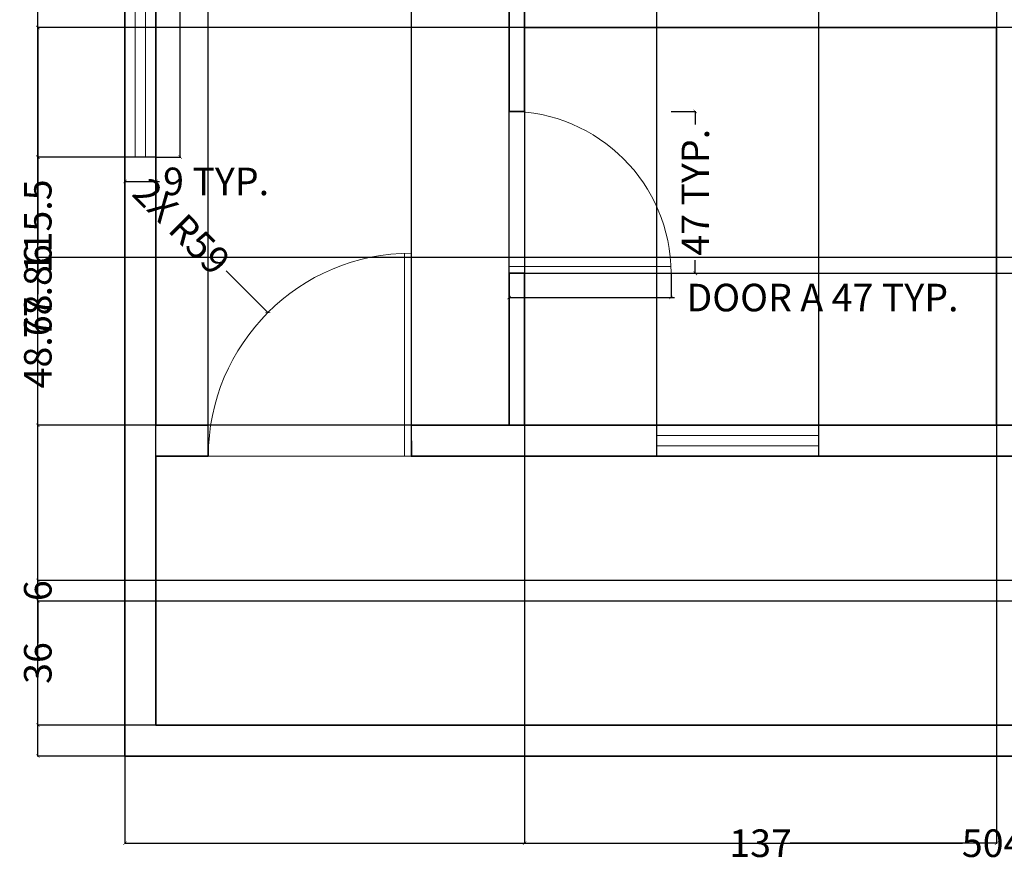
# Model space of a CAD drawing. Units: inches. Extents: x 878 to 1443, y 634 to 1188.
# Tile 1 of 5: x 878 to 1164, y 634 to 878. Entities that reach past the tile are written whole.
import ezdxf

# ---------------------------------------------------------------- set-up
doc = ezdxf.new("R2010")
doc.units = ezdxf.units.IN
doc.header["$MEASUREMENT"] = 0
doc.layers.add('A-ANNO-DIMS', color=2, linetype='Continuous', lineweight=18)
doc.layers.add('A-WALL', color=7, linetype='Continuous', lineweight=35)
doc.layers.add('A-DOOR', color=41, linetype='Continuous', lineweight=18, true_color=0xf4ee51)
doc.layers.add('A-GLAZ', color=152, linetype='Continuous', lineweight=18, true_color=0x2776bb)
doc.styles.get("Standard").update_dxf_attribs({"font": 'arial.ttf'})
doc.dimstyles.get("Standard").update_dxf_attribs({"dimtxt": 8, "dimasz": 1, "dimexe": 0.18, "dimexo": 0.0625, "dimgap": 0.09, "dimtad": 0, "dimdec": 4, "dimzin": 0, "dimdsep": 46, "dimlunit": 3, "dimtxsty": 'Standard', "dimblk": 'ARCHTICK', "dimcen": 0.09, "dimclrd": 6, "dimclre": 5, "dimclrt": 140, "dimadec": 0, "dimazin": 0, "dimtfac": 1, "dimtdec": 4, "dimtofl": 0, "dimtmove": 0, "dimatfit": 3, "dimfxl": 1, "dimtolj": 1, "dimtzin": 0, "dimarcsym": 0})

# ---------------------------------------------------------------- blocks, each defined once
blk = doc.blocks.new('WIN-47IN')
for p, q in [((9, 47), (0, 47)), ((0, 47), (0, 0)), ((3, 0), (3, 47)), ((6, 0), (6, 47)), ((9, 0), (9, 47)), ((0, 0), (9, 0))]:
    blk.add_line(p, q)
blk = doc.blocks.new('DOOR-47IN')
for p, q in [((0, 47), (0, 0)), ((0, 2), (46.96, 2)), ((0, 0), (47, 0))]:
    blk.add_line(p, q)
blk.add_arc((0, 0), 47, 0, 90)
blk = doc.blocks.new('DOOR-59IN')
for p, q in [((57, 0), (57, 58.97)), ((59, 0), (59, 59)), ((0, 0), (59, 0))]:
    blk.add_line(p, q)
blk.add_arc((59, 0), 59, 90, 180)
blk = doc.blocks.new('_ArchTick')
at = {"color": 0, "linetype": 'ByBlock', "const_width": 0.15}
blk.add_lwpolyline([(-0.5, -0.5), (0.5, 0.5)], dxfattribs=at)
blk = doc.blocks.new('*D9')
at = {"layer": 'A-ANNO-DIMS', "color": 6, "lineweight": -2, "transparency": 16777216}
for p, q in [((924.95, 885.33), (924.95, 886.33)), ((924.95, 838.33), (924.95, 885.33))]:
    blk.add_line(p, q, dxfattribs=at)
at = {"layer": 'A-ANNO-DIMS', "color": 5, "lineweight": -2, "transparency": 16777216}
for p, q in [((917.96, 885.33), (925.13, 885.33)), ((917.96, 838.33), (925.13, 838.33))]:
    blk.add_line(p, q, dxfattribs=at)
at = {"layer": 'Defpoints', "color": 0, "lineweight": -2, "transparency": 16777216}
for p in [(917.9, 885.33), (924.95, 885.33), (917.9, 838.33)]:
    blk.add_point(p, dxfattribs=at)
at = {"layer": 'A-ANNO-DIMS', "color": 6, "lineweight": -2, "transparency": 16777216}
for p, rotation in [((924.95, 885.33), 90), ((924.95, 838.33), 270)]:
    blk.add_blockref('_ArchTick', p, dxfattribs=dict(at, rotation=rotation))
at = {"layer": 'A-ANNO-DIMS', "color": 140, "transparency": 16777216, "insert": (924.95, 937.4), "char_height": 8, "attachment_point": 5, "rotation": 90}
blk.add_mtext('\\A1;WINDOW A 47 TYP.', dxfattribs=at)
blk = doc.blocks.new('*D10')
at = {"layer": 'A-ANNO-DIMS', "color": 5, "lineweight": -2, "transparency": 16777216}
for p, q in [((908.9, 838.26), (908.9, 831.1)), ((917.9, 838.26), (917.9, 831.1))]:
    blk.add_line(p, q, dxfattribs=at)
at = {"layer": 'A-ANNO-DIMS', "color": 6, "lineweight": -2, "transparency": 16777216}
for p, q in [((908.9, 831.28), (917.9, 831.28)), ((917.9, 831.28), (918.9, 831.28))]:
    blk.add_line(p, q, dxfattribs=at)
at = {"layer": 'Defpoints', "color": 0, "lineweight": -2, "transparency": 16777216}
for p in [(908.9, 838.33), (917.9, 838.33), (917.9, 831.28)]:
    blk.add_point(p, dxfattribs=at)
at = {"layer": 'A-ANNO-DIMS', "color": 6, "lineweight": -2, "transparency": 16777216, "rotation": 180}
blk.add_blockref('_ArchTick', (908.9, 831.28), dxfattribs=at)
at = {"layer": 'A-ANNO-DIMS', "color": 6, "lineweight": -2, "transparency": 16777216}
blk.add_blockref('_ArchTick', (917.9, 831.28), dxfattribs=at)
at = {"layer": 'A-ANNO-DIMS', "color": 140, "transparency": 16777216, "insert": (935.35, 831.28), "char_height": 8, "attachment_point": 5}
blk.add_mtext('\\A1;9 TYP.', dxfattribs=at)
blk = doc.blocks.new('*D15')
at = {"layer": 'A-ANNO-DIMS', "color": 5, "lineweight": -2, "transparency": 16777216}
for p, q in [((1020.4, 804.54), (1020.4, 797.38)), ((1067.4, 804.54), (1067.4, 797.38))]:
    blk.add_line(p, q, dxfattribs=at)
at = {"layer": 'A-ANNO-DIMS', "color": 6, "lineweight": -2, "transparency": 16777216}
for p, q in [((1020.4, 797.56), (1067.4, 797.56)), ((1067.4, 797.56), (1068.4, 797.56))]:
    blk.add_line(p, q, dxfattribs=at)
at = {"layer": 'Defpoints', "color": 0, "lineweight": -2, "transparency": 16777216}
for p in [(1020.4, 804.61), (1067.4, 804.61), (1067.4, 797.56)]:
    blk.add_point(p, dxfattribs=at)
at = {"layer": 'A-ANNO-DIMS', "color": 6, "lineweight": -2, "transparency": 16777216, "rotation": 180}
blk.add_blockref('_ArchTick', (1020.4, 797.56), dxfattribs=at)
at = {"layer": 'A-ANNO-DIMS', "color": 6, "lineweight": -2, "transparency": 16777216}
blk.add_blockref('_ArchTick', (1067.4, 797.56), dxfattribs=at)
at = {"layer": 'A-ANNO-DIMS', "color": 140, "transparency": 16777216, "insert": (1111.36, 797.56), "char_height": 8, "attachment_point": 5}
blk.add_mtext('\\A1;DOOR A 47 TYP.', dxfattribs=at)
blk = doc.blocks.new('*D16')
at = {"layer": 'A-ANNO-DIMS', "color": 5, "lineweight": -2, "transparency": 16777216}
for p, q in [((1067.46, 851.61), (1074.63, 851.61)), ((1067.46, 804.61), (1074.63, 804.61))]:
    blk.add_line(p, q, dxfattribs=at)
at = {"layer": 'A-ANNO-DIMS', "color": 6, "lineweight": -2, "transparency": 16777216}
for p, q in [((1074.45, 851.61), (1074.45, 847.83)), ((1074.45, 804.61), (1074.45, 808.39))]:
    blk.add_line(p, q, dxfattribs=at)
at = {"layer": 'Defpoints', "color": 0, "lineweight": -2, "transparency": 16777216}
for p in [(1067.4, 851.61), (1074.45, 851.61), (1067.4, 804.61)]:
    blk.add_point(p, dxfattribs=at)
at = {"layer": 'A-ANNO-DIMS', "color": 6, "lineweight": -2, "transparency": 16777216}
for p, rotation in [((1074.45, 851.61), 90), ((1074.45, 804.61), 270)]:
    blk.add_blockref('_ArchTick', p, dxfattribs=dict(at, rotation=rotation))
at = {"layer": 'A-ANNO-DIMS', "color": 140, "transparency": 16777216, "insert": (1074.45, 828.11), "char_height": 8, "attachment_point": 5, "rotation": 90}
blk.add_mtext('\\A1;47 TYP.', dxfattribs=at)
blk = doc.blocks.new('*D21')
at = {"layer": 'A-ANNO-DIMS', "color": 5, "lineweight": -2, "transparency": 16777216}
for p, q in [((908.9, 664.41), (908.9, 638.98)), ((1412.9, 664.41), (1412.9, 638.98))]:
    blk.add_line(p, q, dxfattribs=at)
at = {"layer": 'A-ANNO-DIMS', "color": 6, "lineweight": -2, "transparency": 16777216}
for p, q in [((908.9, 639.16), (1151.99, 639.16)), ((1412.9, 639.16), (1169.81, 639.16))]:
    blk.add_line(p, q, dxfattribs=at)
at = {"layer": 'Defpoints', "color": 0, "lineweight": -2, "transparency": 16777216}
for p in [(908.9, 664.47), (1412.9, 664.47), (1412.9, 639.16)]:
    blk.add_point(p, dxfattribs=at)
at = {"layer": 'A-ANNO-DIMS', "color": 6, "lineweight": -2, "transparency": 16777216, "rotation": 180}
blk.add_blockref('_ArchTick', (908.9, 639.16), dxfattribs=at)
at = {"layer": 'A-ANNO-DIMS', "color": 6, "lineweight": -2, "transparency": 16777216}
blk.add_blockref('_ArchTick', (1412.9, 639.16), dxfattribs=at)
at = {"layer": 'A-ANNO-DIMS', "color": 140, "transparency": 16777216, "insert": (1160.9, 639.16), "char_height": 8, "attachment_point": 5}
blk.add_mtext('\\A1;504', dxfattribs=at)
blk = doc.blocks.new('*D22')
at = {"layer": 'A-ANNO-DIMS', "color": 5, "lineweight": -2, "transparency": 16777216}
for p, q in [((908.84, 1120.47), (883.41, 1120.47)), ((908.84, 664.47), (883.41, 664.47))]:
    blk.add_line(p, q, dxfattribs=at)
at = {"layer": 'A-ANNO-DIMS', "color": 6, "lineweight": -2, "transparency": 16777216}
for p, q in [((883.59, 1120.47), (883.59, 901.56)), ((883.59, 664.47), (883.59, 883.38))]:
    blk.add_line(p, q, dxfattribs=at)
at = {"layer": 'Defpoints', "color": 0, "lineweight": -2, "transparency": 16777216}
for p in [(883.59, 1120.47), (908.9, 1120.47), (908.9, 664.47)]:
    blk.add_point(p, dxfattribs=at)
at = {"layer": 'A-ANNO-DIMS', "color": 6, "lineweight": -2, "transparency": 16777216}
for p, rotation in [((883.59, 1120.47), 90), ((883.59, 664.47), 270)]:
    blk.add_blockref('_ArchTick', p, dxfattribs=dict(at, rotation=rotation))
at = {"layer": 'A-ANNO-DIMS', "color": 140, "transparency": 16777216, "insert": (883.59, 892.47), "char_height": 8, "attachment_point": 5, "rotation": 90}
blk.add_mtext('\\A1;456', dxfattribs=at)
blk = doc.blocks.new('*D28')
at = {"layer": 'A-ANNO-DIMS', "color": 5, "lineweight": -2, "transparency": 16777216}
for p, q in [((917.84, 838.33), (883.41, 838.33)), ((917.84, 760.47), (883.41, 760.47))]:
    blk.add_line(p, q, dxfattribs=at)
at = {"layer": 'A-ANNO-DIMS', "color": 6, "lineweight": -2, "transparency": 16777216}
for p, q in [((883.59, 838.33), (883.59, 812.95)), ((883.59, 760.47), (883.59, 785.85))]:
    blk.add_line(p, q, dxfattribs=at)
at = {"layer": 'Defpoints', "color": 0, "lineweight": -2, "transparency": 16777216}
for p in [(883.59, 838.33), (917.9, 838.33), (917.9, 760.47)]:
    blk.add_point(p, dxfattribs=at)
at = {"layer": 'A-ANNO-DIMS', "color": 6, "lineweight": -2, "transparency": 16777216}
for p, rotation in [((883.59, 838.33), 90), ((883.59, 760.47), 270)]:
    blk.add_blockref('_ArchTick', p, dxfattribs=dict(at, rotation=rotation))
at = {"layer": 'A-ANNO-DIMS', "color": 140, "transparency": 16777216, "insert": (883.59, 799.4), "char_height": 8, "attachment_point": 5, "rotation": 90}
blk.add_mtext('\\A1;77.86', dxfattribs=at)
blk = doc.blocks.new('*D33')
at = {"layer": 'A-ANNO-DIMS', "color": 5, "lineweight": -2, "transparency": 16777216}
for p, q in [((917.9, 760.53), (917.9, 1145.96)), ((1020.4, 760.53), (1020.4, 1145.96))]:
    blk.add_line(p, q, dxfattribs=at)
at = {"layer": 'A-ANNO-DIMS', "color": 6, "lineweight": -2, "transparency": 16777216}
for p, q in [((917.9, 1145.78), (955.91, 1145.78)), ((1020.4, 1145.78), (982.39, 1145.78))]:
    blk.add_line(p, q, dxfattribs=at)
at = {"layer": 'Defpoints', "color": 0, "lineweight": -2, "transparency": 16777216}
for p in [(1020.4, 1145.78), (917.9, 760.47), (1020.4, 760.47)]:
    blk.add_point(p, dxfattribs=at)
at = {"layer": 'A-ANNO-DIMS', "color": 6, "lineweight": -2, "transparency": 16777216, "rotation": 180}
blk.add_blockref('_ArchTick', (917.9, 1145.78), dxfattribs=at)
at = {"layer": 'A-ANNO-DIMS', "color": 6, "lineweight": -2, "transparency": 16777216}
blk.add_blockref('_ArchTick', (1020.4, 1145.78), dxfattribs=at)
at = {"layer": 'A-ANNO-DIMS', "color": 140, "transparency": 16777216, "insert": (969.15, 1145.78), "char_height": 8, "attachment_point": 5}
blk.add_mtext('\\A1;102.5', dxfattribs=at)
blk = doc.blocks.new('*D34')
at = {"layer": 'A-ANNO-DIMS', "color": 5, "lineweight": -2, "transparency": 16777216}
for p, q in [((1024.9, 1111.41), (1024.9, 638.98)), ((1161.9, 1111.41), (1161.9, 638.98))]:
    blk.add_line(p, q, dxfattribs=at)
at = {"layer": 'A-ANNO-DIMS', "color": 6, "lineweight": -2, "transparency": 16777216}
for p, q in [((1024.9, 639.16), (1084.85, 639.16)), ((1161.9, 639.16), (1101.95, 639.16))]:
    blk.add_line(p, q, dxfattribs=at)
at = {"layer": 'Defpoints', "color": 0, "lineweight": -2, "transparency": 16777216}
for p in [(1024.9, 1111.47), (1161.9, 1111.47), (1161.9, 639.16)]:
    blk.add_point(p, dxfattribs=at)
at = {"layer": 'A-ANNO-DIMS', "color": 6, "lineweight": -2, "transparency": 16777216, "rotation": 180}
blk.add_blockref('_ArchTick', (1024.9, 639.16), dxfattribs=at)
at = {"layer": 'A-ANNO-DIMS', "color": 6, "lineweight": -2, "transparency": 16777216}
blk.add_blockref('_ArchTick', (1161.9, 639.16), dxfattribs=at)
at = {"layer": 'A-ANNO-DIMS', "color": 140, "transparency": 16777216, "insert": (1093.4, 639.16), "char_height": 8, "attachment_point": 5}
blk.add_mtext('\\A1;137', dxfattribs=at)
blk = doc.blocks.new('*D38')
at = {"layer": 'A-ANNO-DIMS', "color": 5, "lineweight": -2, "transparency": 16777216}
for p, q in [((1403.84, 875.97), (883.41, 875.97)), ((1403.84, 760.47), (883.41, 760.47))]:
    blk.add_line(p, q, dxfattribs=at)
at = {"layer": 'A-ANNO-DIMS', "color": 6, "lineweight": -2, "transparency": 16777216}
for p, q in [((883.59, 875.97), (883.59, 831.46)), ((883.59, 760.47), (883.59, 804.98))]:
    blk.add_line(p, q, dxfattribs=at)
at = {"layer": 'Defpoints', "color": 0, "lineweight": -2, "transparency": 16777216}
for p in [(1403.9, 875.97), (883.59, 760.47), (1403.9, 760.47)]:
    blk.add_point(p, dxfattribs=at)
at = {"layer": 'A-ANNO-DIMS', "color": 6, "lineweight": -2, "transparency": 16777216}
for p, rotation in [((883.59, 875.97), 90), ((883.59, 760.47), 270)]:
    blk.add_blockref('_ArchTick', p, dxfattribs=dict(at, rotation=rotation))
at = {"layer": 'A-ANNO-DIMS', "color": 140, "transparency": 16777216, "insert": (883.59, 818.22), "char_height": 8, "attachment_point": 5, "rotation": 90}
blk.add_mtext('\\A1;115.5', dxfattribs=at)
blk = doc.blocks.new('*D44')
at = {"layer": 'A-ANNO-DIMS', "color": 5, "lineweight": -2, "transparency": 16777216}
for p, q in [((917.9, 751.53), (917.9, 1145.96)), ((933.09, 751.53), (933.09, 1145.96))]:
    blk.add_line(p, q, dxfattribs=at)
at = {"layer": 'A-ANNO-DIMS', "color": 6, "lineweight": -2, "transparency": 16777216}
for p, q in [((917.9, 1145.78), (933.09, 1145.78)), ((933.09, 1145.78), (934.09, 1145.78))]:
    blk.add_line(p, q, dxfattribs=at)
at = {"layer": 'Defpoints', "color": 0, "lineweight": -2, "transparency": 16777216}
for p in [(933.09, 1145.78), (917.9, 751.47), (933.09, 751.47)]:
    blk.add_point(p, dxfattribs=at)
at = {"layer": 'A-ANNO-DIMS', "color": 6, "lineweight": -2, "transparency": 16777216, "rotation": 180}
blk.add_blockref('_ArchTick', (917.9, 1145.78), dxfattribs=at)
at = {"layer": 'A-ANNO-DIMS', "color": 6, "lineweight": -2, "transparency": 16777216}
blk.add_blockref('_ArchTick', (933.09, 1145.78), dxfattribs=at)
at = {"layer": 'A-ANNO-DIMS', "color": 140, "transparency": 16777216, "insert": (950.4, 1145.78), "char_height": 8, "attachment_point": 5}
blk.add_mtext('\\A1;15.187', dxfattribs=at)
blk = doc.blocks.new('*D45')
at = {"layer": 'A-ANNO-DIMS', "color": 5, "lineweight": -2, "transparency": 16777216}
for p, q in [((992.09, 751.53), (992.09, 1145.96)), ((1063.3, 751.53), (1063.3, 1145.96))]:
    blk.add_line(p, q, dxfattribs=at)
at = {"layer": 'A-ANNO-DIMS', "color": 6, "lineweight": -2, "transparency": 16777216}
for p, q in [((992.09, 1145.78), (1014.18, 1145.78)), ((1063.3, 1145.78), (1041.21, 1145.78))]:
    blk.add_line(p, q, dxfattribs=at)
at = {"layer": 'Defpoints', "color": 0, "lineweight": -2, "transparency": 16777216}
for p in [(1063.3, 1145.78), (992.09, 751.47), (1063.3, 751.47)]:
    blk.add_point(p, dxfattribs=at)
at = {"layer": 'A-ANNO-DIMS', "color": 6, "lineweight": -2, "transparency": 16777216, "rotation": 180}
blk.add_blockref('_ArchTick', (992.09, 1145.78), dxfattribs=at)
at = {"layer": 'A-ANNO-DIMS', "color": 6, "lineweight": -2, "transparency": 16777216}
blk.add_blockref('_ArchTick', (1063.3, 1145.78), dxfattribs=at)
at = {"layer": 'A-ANNO-DIMS', "color": 140, "transparency": 16777216, "insert": (1027.69, 1145.78), "char_height": 8, "attachment_point": 5}
blk.add_mtext('\\A1;71.22', dxfattribs=at)
blk = doc.blocks.new('*D46')
at = {"layer": 'A-ANNO-DIMS', "color": 5, "lineweight": -2, "transparency": 16777216}
for p, q in [((1110.3, 751.53), (1110.3, 1145.96)), ((1172.39, 751.53), (1172.39, 1145.96))]:
    blk.add_line(p, q, dxfattribs=at)
at = {"layer": 'A-ANNO-DIMS', "color": 6, "lineweight": -2, "transparency": 16777216}
for p, q in [((1110.3, 1145.78), (1127.73, 1145.78)), ((1172.39, 1145.78), (1154.96, 1145.78))]:
    blk.add_line(p, q, dxfattribs=at)
at = {"layer": 'Defpoints', "color": 0, "lineweight": -2, "transparency": 16777216}
for p in [(1172.39, 1145.78), (1110.3, 751.47), (1172.39, 751.47)]:
    blk.add_point(p, dxfattribs=at)
at = {"layer": 'A-ANNO-DIMS', "color": 6, "lineweight": -2, "transparency": 16777216, "rotation": 180}
blk.add_blockref('_ArchTick', (1110.3, 1145.78), dxfattribs=at)
at = {"layer": 'A-ANNO-DIMS', "color": 6, "lineweight": -2, "transparency": 16777216}
blk.add_blockref('_ArchTick', (1172.39, 1145.78), dxfattribs=at)
at = {"layer": 'A-ANNO-DIMS', "color": 140, "transparency": 16777216, "insert": (1141.35, 1145.78), "char_height": 8, "attachment_point": 5}
blk.add_mtext('\\A1;62.08', dxfattribs=at)
blk = doc.blocks.new('*D47')
at = {"layer": 'A-ANNO-DIMS', "color": 5, "lineweight": -2, "transparency": 16777216}
for p, q in [((1020.46, 804.61), (1438.39, 804.61)), ((1020.46, 760.47), (1438.39, 760.47))]:
    blk.add_line(p, q, dxfattribs=at)
at = {"layer": 'A-ANNO-DIMS', "color": 6, "lineweight": -2, "transparency": 16777216}
for p, q in [((1438.21, 804.61), (1438.21, 796.27)), ((1438.21, 760.47), (1438.21, 768.81))]:
    blk.add_line(p, q, dxfattribs=at)
at = {"layer": 'Defpoints', "color": 0, "lineweight": -2, "transparency": 16777216}
for p in [(1020.4, 804.61), (1438.21, 804.61), (1020.4, 760.47)]:
    blk.add_point(p, dxfattribs=at)
at = {"layer": 'A-ANNO-DIMS', "color": 6, "lineweight": -2, "transparency": 16777216}
for p, rotation in [((1438.21, 804.61), 90), ((1438.21, 760.47), 270)]:
    blk.add_blockref('_ArchTick', p, dxfattribs=dict(at, rotation=rotation))
at = {"layer": 'A-ANNO-DIMS', "color": 140, "transparency": 16777216, "insert": (1438.21, 782.54), "char_height": 8, "attachment_point": 5, "rotation": 90}
blk.add_mtext('\\A1;44.14', dxfattribs=at)
blk = doc.blocks.new('*D48')
at = {"layer": 'A-ANNO-DIMS', "color": 5, "lineweight": -2, "transparency": 16777216}
for p, q in [((1262.34, 809.15), (883.41, 809.15)), ((1262.34, 760.47), (883.41, 760.47))]:
    blk.add_line(p, q, dxfattribs=at)
at = {"layer": 'A-ANNO-DIMS', "color": 6, "lineweight": -2, "transparency": 16777216}
for p, q in [((883.59, 809.15), (883.59, 798.57)), ((883.59, 760.47), (883.59, 771.05))]:
    blk.add_line(p, q, dxfattribs=at)
at = {"layer": 'Defpoints', "color": 0, "lineweight": -2, "transparency": 16777216}
for p in [(883.59, 809.15), (1262.4, 809.15), (1262.4, 760.47)]:
    blk.add_point(p, dxfattribs=at)
at = {"layer": 'A-ANNO-DIMS', "color": 6, "lineweight": -2, "transparency": 16777216}
for p, rotation in [((883.59, 809.15), 90), ((883.59, 760.47), 270)]:
    blk.add_blockref('_ArchTick', p, dxfattribs=dict(at, rotation=rotation))
at = {"layer": 'A-ANNO-DIMS', "color": 140, "transparency": 16777216, "insert": (883.59, 784.81), "char_height": 8, "attachment_point": 5, "rotation": 90}
blk.add_mtext('\\A1;48.68', dxfattribs=at)
blk = doc.blocks.new('*D60')
at = {"layer": 'A-ANNO-DIMS', "color": 5, "lineweight": -2, "transparency": 16777216}
for p, q in [((1247.84, 709.47), (883.41, 709.47)), ((1247.84, 673.47), (883.41, 673.47))]:
    blk.add_line(p, q, dxfattribs=at)
at = {"layer": 'A-ANNO-DIMS', "color": 6, "lineweight": -2, "transparency": 16777216}
for p, q in [((883.59, 709.47), (883.59, 697.28)), ((883.59, 673.47), (883.59, 685.66))]:
    blk.add_line(p, q, dxfattribs=at)
at = {"layer": 'Defpoints', "color": 0, "lineweight": -2, "transparency": 16777216}
for p in [(883.59, 709.47), (1247.9, 709.47), (1247.9, 673.47)]:
    blk.add_point(p, dxfattribs=at)
at = {"layer": 'A-ANNO-DIMS', "color": 6, "lineweight": -2, "transparency": 16777216}
for p, rotation in [((883.59, 709.47), 90), ((883.59, 673.47), 270)]:
    blk.add_blockref('_ArchTick', p, dxfattribs=dict(at, rotation=rotation))
at = {"layer": 'A-ANNO-DIMS', "color": 140, "transparency": 16777216, "insert": (883.59, 691.47), "char_height": 8, "attachment_point": 5, "rotation": 90}
blk.add_mtext('\\A1;36', dxfattribs=at)
blk = doc.blocks.new('*D61')
at = {"layer": 'A-ANNO-DIMS', "color": 5, "lineweight": -2, "transparency": 16777216}
for p, q in [((1247.84, 715.47), (883.41, 715.47)), ((1247.84, 709.47), (883.41, 709.47))]:
    blk.add_line(p, q, dxfattribs=at)
at = {"layer": 'A-ANNO-DIMS', "color": 6, "lineweight": -2, "transparency": 16777216}
for p, q in [((883.59, 715.47), (883.59, 715.2)), ((883.59, 709.47), (883.59, 709.74))]:
    blk.add_line(p, q, dxfattribs=at)
at = {"layer": 'Defpoints', "color": 0, "lineweight": -2, "transparency": 16777216}
for p in [(883.59, 715.47), (1247.9, 715.47), (1247.9, 709.47)]:
    blk.add_point(p, dxfattribs=at)
at = {"layer": 'A-ANNO-DIMS', "color": 6, "lineweight": -2, "transparency": 16777216}
for p, rotation in [((883.59, 715.47), 90), ((883.59, 709.47), 270)]:
    blk.add_blockref('_ArchTick', p, dxfattribs=dict(at, rotation=rotation))
at = {"layer": 'A-ANNO-DIMS', "color": 140, "transparency": 16777216, "insert": (883.59, 712.47), "char_height": 8, "attachment_point": 5, "rotation": 90}
blk.add_mtext('\\A1;6', dxfattribs=at)
blk = doc.blocks.new('*D63')
at = {"layer": 'A-ANNO-DIMS', "color": 5, "lineweight": -2, "transparency": 16777216}
for p, q in [((1020.4, 851.67), (1020.4, 1145.96)), ((1024.9, 851.67), (1024.9, 1145.96))]:
    blk.add_line(p, q, dxfattribs=at)
at = {"layer": 'A-ANNO-DIMS', "color": 6, "lineweight": -2, "transparency": 16777216}
for p, q in [((1020.4, 1145.78), (1024.9, 1145.78)), ((1024.9, 1145.78), (1025.9, 1145.78))]:
    blk.add_line(p, q, dxfattribs=at)
at = {"layer": 'Defpoints', "color": 0, "lineweight": -2, "transparency": 16777216}
for p in [(1024.9, 1145.78), (1020.4, 851.61), (1024.9, 851.61)]:
    blk.add_point(p, dxfattribs=at)
at = {"layer": 'A-ANNO-DIMS', "color": 6, "lineweight": -2, "transparency": 16777216, "rotation": 180}
blk.add_blockref('_ArchTick', (1020.4, 1145.78), dxfattribs=at)
at = {"layer": 'A-ANNO-DIMS', "color": 6, "lineweight": -2, "transparency": 16777216}
blk.add_blockref('_ArchTick', (1024.9, 1145.78), dxfattribs=at)
at = {"layer": 'A-ANNO-DIMS', "color": 140, "transparency": 16777216, "insert": (1033.46, 1145.78), "char_height": 8, "attachment_point": 5}
blk.add_mtext('\\A1;4.5', dxfattribs=at)
blk = doc.blocks.new('*D68')
at = {"layer": 'A-ANNO-DIMS', "color": 6, "lineweight": -2, "transparency": 16777216}
blk.add_line((938.29, 805.27), (950.37, 793.19), dxfattribs=at)
at = {"layer": 'A-ANNO-DIMS', "color": 5, "lineweight": -2, "transparency": 16777216}
for p, q in [((992, 751.47), (992.18, 751.47)), ((992.09, 751.38), (992.09, 751.56))]:
    blk.add_line(p, q, dxfattribs=at)
at = {"layer": 'Defpoints', "color": 0, "lineweight": -2, "transparency": 16777216}
for p in [(950.37, 793.19), (992.09, 751.47)]:
    blk.add_point(p, dxfattribs=at)
at = {"layer": 'A-ANNO-DIMS', "color": 6, "lineweight": -2, "transparency": 16777216, "rotation": 315.0003563879212}
blk.add_blockref('_ArchTick', (950.37, 793.19), dxfattribs=at)
at = {"layer": 'A-ANNO-DIMS', "color": 140, "transparency": 16777216, "insert": (925.33, 818.22), "char_height": 8, "attachment_point": 5, "rotation": 315.0004}
blk.add_mtext('\\A1;2X R59', dxfattribs=at)

msp = doc.modelspace()

# ---------------------------------------------------------------- linework, layer by layer
at = {"layer": 'A-WALL'}
for p, q in [((908.8987, 664.4702), (908.8987, 1120.4702)), ((917.8987, 760.4702), (917.8987, 968.9702)), ((1020.3987, 936.5702), (1020.3987, 851.6074)), ((1161.8987, 875.9702), (1024.8987, 875.9702)), ((1024.8987, 875.9702), (1024.8987, 851.6074)), ((1161.8987, 875.9702), (1161.8987, 760.4702)), ((1020.3987, 851.6074), (1024.8987, 851.6074)), ((1020.3987, 804.6074), (1024.8987, 804.6074)), ((1020.3987, 804.6074), (1020.3987, 760.4702)), ((1024.8987, 804.6074), (1024.8987, 760.4702)), ((933.0853, 760.4702), (917.8987, 760.4702)), ((1020.3987, 760.4702), (992.0853, 760.4702)), ((1161.8987, 760.4702), (1024.8987, 760.4702)), ((933.0853, 755.9702), (933.0853, 751.4702)), ((992.0853, 755.9702), (992.0853, 751.4702)), ((917.8987, 673.4702), (917.8987, 751.4702)), ((933.0853, 751.4702), (917.8987, 751.4702)), ((1172.3876, 751.4702), (992.0853, 751.4702)), ((1403.8987, 673.4702), (917.8987, 673.4702)), ((1412.8987, 664.4702), (908.8987, 664.4702))]:
    msp.add_line(p, q, dxfattribs=at)

# ---------------------------------------------------------------- block references
at = {"layer": 'A-DOOR'}
for name, p in [('DOOR-47IN', (1020.3987, 804.6074)), ('DOOR-59IN', (933.0853, 751.4702))]:
    msp.add_blockref(name, p, dxfattribs=at)
at = {"layer": 'A-GLAZ'}
msp.add_blockref('WIN-47IN', (908.8987, 838.3253), dxfattribs=at)
at = {"layer": 'A-GLAZ', "rotation": 269.9999999999992}
msp.add_blockref('WIN-47IN', (1063.3038, 760.4702), dxfattribs=at)

# ---------------------------------------------------------------- dimensions: what is measured, and where the dimension line sits
at = {"layer": 'A-ANNO-DIMS'}
for base, p1, p2, override, picture, middle in [((1020.3987, 1145.7802), (917.8987, 760.4702), (1020.3987, 760.4702), {"dimdec": 1, "dimlfac": 1, "dimrnd": 0, "dimzin": 0, "dimdsep": 46, "dimlunit": 2}, '*D33', (969.1487, 1145.7802)), ((933.0853, 1145.7802), (917.8987, 751.4702), (933.0853, 751.4702), {"dimdec": 3, "dimlfac": 1, "dimrnd": 0, "dimzin": 0, "dimdsep": 46, "dimlunit": 2}, '*D44', (950.4045, 1145.7802)), ((1063.3038, 1145.7802), (992.0853, 751.4702), (1063.3038, 751.4702), {"dimdec": 2, "dimlfac": 1, "dimrnd": 0, "dimzin": 0, "dimdsep": 46, "dimlunit": 2}, '*D45', (1027.6946, 1145.7802)), ((1024.8987, 1145.7802), (1020.3987, 851.6074), (1024.8987, 851.6074), {"dimdec": 1, "dimlfac": 1, "dimrnd": 0, "dimzin": 0, "dimdsep": 46, "dimlunit": 2}, '*D63', (1033.462, 1145.7802)), ((1172.3876, 1145.7802), (1110.3038, 751.4702), (1172.3876, 751.4702), {"dimdec": 2, "dimlfac": 1, "dimrnd": 0, "dimzin": 0, "dimdsep": 46, "dimlunit": 2}, '*D46', (1141.3457, 1145.7802)), ((1161.8987, 639.1602), (1024.8987, 1111.4702), (1161.8987, 1111.4702), {"dimdec": 0, "dimlfac": 1, "dimrnd": 0, "dimzin": 0, "dimdsep": 46, "dimlunit": 2}, '*D34', (1093.3987, 639.1602)), ((1412.8987, 639.1602), (908.8987, 664.4702), (1412.8987, 664.4702), {"dimdec": 0, "dimlfac": 1, "dimrnd": 0, "dimzin": 0, "dimdsep": 46, "dimlunit": 2}, '*D21', (1160.8987, 639.1602))]:
    dim = msp.add_linear_dim(base=base, p1=p1, p2=p2, dimstyle='Standard', override=override, dxfattribs=at)
    dim.commit()
    dim.dimension.update_dxf_attribs({"geometry": picture, "text_midpoint": middle})
for base, p1, p2, override, picture, middle in [((883.5887, 1120.4702), (908.8987, 664.4702), (908.8987, 1120.4702), {"dimdec": 0, "dimlfac": 1, "dimrnd": 0, "dimzin": 0, "dimdsep": 46, "dimlunit": 2}, '*D22', (883.5887, 892.4702)), ((883.5887, 760.4702), (1403.8987, 875.9702), (1403.8987, 760.4702), {"dimdec": 1, "dimlfac": 1, "dimrnd": 0, "dimzin": 0, "dimdsep": 46, "dimlunit": 2}, '*D38', (883.5887, 818.2202)), ((883.5887, 838.3253), (917.8987, 760.4702), (917.8987, 838.3253), {"dimdec": 2, "dimlfac": 1, "dimrnd": 0, "dimzin": 0, "dimdsep": 46, "dimlunit": 2}, '*D28', (883.5887, 799.3978)), ((883.5887, 809.1495), (1262.3987, 760.4702), (1262.3987, 809.1495), {"dimdec": 2, "dimlfac": 1, "dimrnd": 0, "dimzin": 0, "dimdsep": 46, "dimlunit": 2}, '*D48', (883.5887, 784.8099)), ((1438.2087, 804.6074), (1020.3987, 760.4702), (1020.3987, 804.6074), {"dimdec": 2, "dimlfac": 1, "dimrnd": 0, "dimzin": 0, "dimdsep": 46, "dimlunit": 2}, '*D47', (1438.2087, 782.5388)), ((883.5887, 715.4702), (1247.8987, 709.4702), (1247.8987, 715.4702), {"dimdec": 0, "dimlfac": 1, "dimrnd": 0, "dimzin": 0, "dimdsep": 46, "dimlunit": 2}, '*D61', (883.5887, 712.4702)), ((883.5887, 709.4702), (1247.8987, 673.4702), (1247.8987, 709.4702), {"dimdec": 0, "dimlfac": 1, "dimrnd": 0, "dimzin": 0, "dimdsep": 46, "dimlunit": 2}, '*D60', (883.5887, 691.4702))]:
    dim = msp.add_linear_dim(base=base, p1=p1, p2=p2, angle=90, dimstyle='Standard', override=override, dxfattribs=at)
    dim.commit()
    dim.dimension.update_dxf_attribs({"geometry": picture, "text_midpoint": middle})
for base, p1, p2, text, picture, middle in [((924.9487, 885.3253), (917.8987, 838.3253), (917.8987, 885.3253), 'WINDOW A <> TYP.', '*D9', (924.9487, 937.4003)), ((1074.4487, 851.6074), (1067.3987, 804.6074), (1067.3987, 851.6074), '<> TYP.', '*D16', (1074.4487, 828.1074))]:
    dim = msp.add_linear_dim(base=base, p1=p1, p2=p2, angle=90, text=text, dimstyle='Standard', override={"dimdec": 0, "dimlfac": 1, "dimrnd": 0, "dimzin": 0, "dimdsep": 46, "dimlunit": 2}, dxfattribs=at)
    dim.commit()
    dim.dimension.update_dxf_attribs({"geometry": picture, "text_midpoint": middle})
for base, p1, p2, text, picture, middle in [((917.8987, 831.2753), (908.8987, 838.3253), (917.8987, 838.3253), '<> TYP.', '*D10', (935.3515, 831.2753)), ((1067.3987, 797.5574), (1020.3987, 804.6074), (1067.3987, 804.6074), 'DOOR A <> TYP.', '*D15', (1111.3563, 797.5574))]:
    dim = msp.add_linear_dim(base=base, p1=p1, p2=p2, text=text, dimstyle='Standard', override={"dimdec": 0, "dimlfac": 1, "dimrnd": 0, "dimzin": 0, "dimdsep": 46, "dimlunit": 2}, dxfattribs=at)
    dim.commit()
    dim.dimension.update_dxf_attribs({"geometry": picture, "text_midpoint": middle})
dim = msp.add_radius_dim(center=(992.0853, 751.4702), mpoint=(950.3658, 793.1892), text='2X <>', dimstyle='Standard', override={"dimdec": 0, "dimlfac": 1, "dimrnd": 0, "dimzin": 0, "dimdsep": 46, "dimlunit": 2}, dxfattribs=at)
dim.commit()
dim.dimension.update_dxf_attribs({"geometry": '*D68', "text_midpoint": (925.334, 818.2207), "dimtype": 164})

doc.saveas('drawing.dxf')
